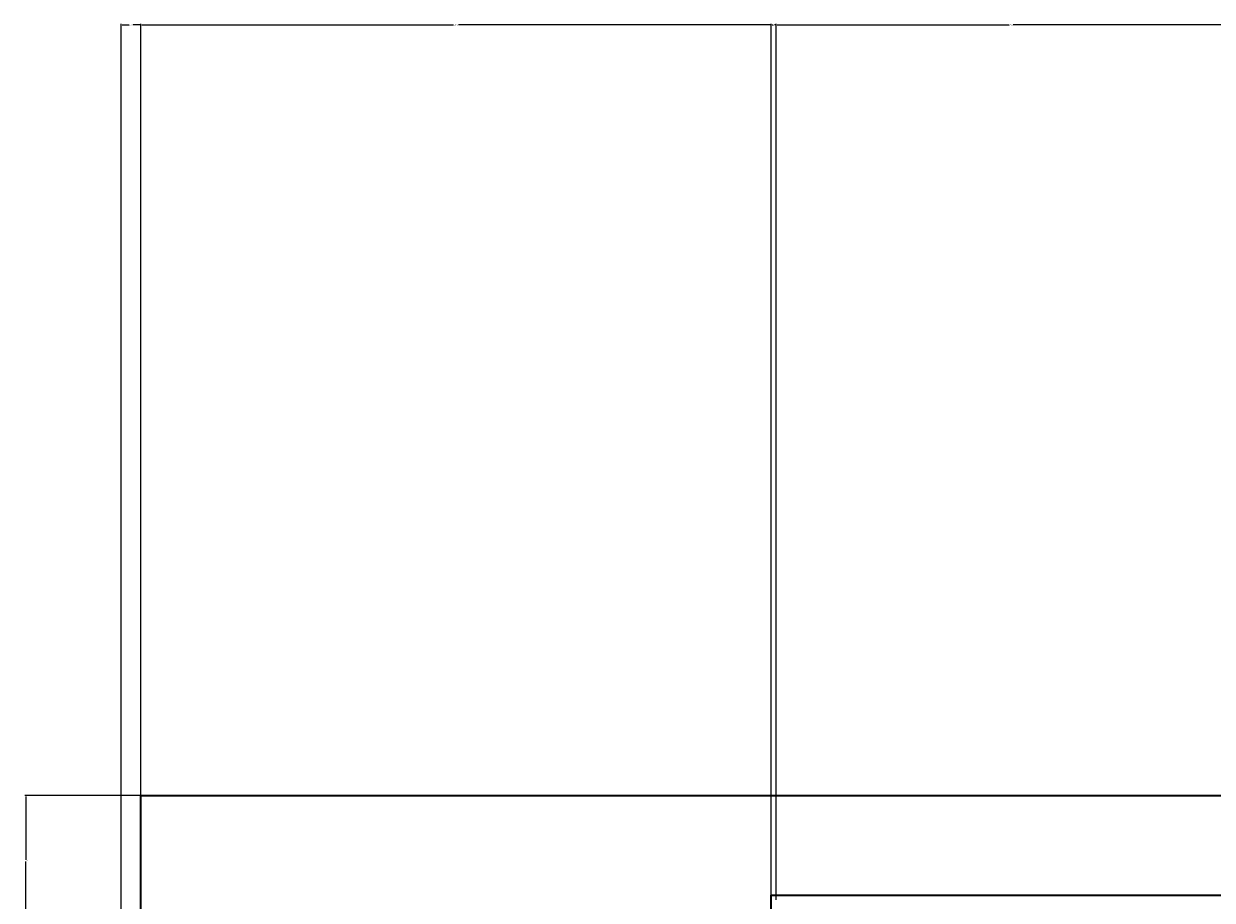
# Model space of a CAD drawing. Units: inches. Extents: x -7 to 391, y -12 to 303.
# Tile 2 of 5: x -7 to 222, y 134 to 303. Entities that reach past the tile are written whole.
import ezdxf

# ---------------------------------------------------------------- set-up
doc = ezdxf.new("R2010")
doc.units = ezdxf.units.IN
doc.header["$MEASUREMENT"] = 0
doc.layers.add('A-ANNO-DIMS', color=2, linetype='Continuous', lineweight=18)
doc.layers.add('A-ELEV', color=7, linetype='Continuous', lineweight=35)
doc.styles.get("Standard").update_dxf_attribs({"font": 'arial.ttf'})
doc.dimstyles.get("Standard").update_dxf_attribs({"dimtxt": 0.18, "dimasz": 0.18, "dimexe": 0.18, "dimexo": 0.0625, "dimgap": 0.09, "dimtad": 0, "dimtih": 1, "dimtoh": 1, "dimdec": 4, "dimzin": 0, "dimdsep": 46, "dimtxsty": 'Standard', "dimcen": 0.09, "dimadec": 0, "dimazin": 0, "dimtfac": 1, "dimtdec": 4, "dimtofl": 0, "dimtmove": 0, "dimatfit": 3, "dimfxl": 1, "dimtolj": 1, "dimtzin": 0, "dimarcsym": 0})

# ---------------------------------------------------------------- blocks, each defined once
blk = doc.blocks.new('*D16')
at = {"layer": 'A-ANNO-DIMS', "color": 0, "lineweight": -2, "transparency": 16777216}
for p, q in [((15.76, 154.35), (-6.56, 154.35)), ((-6.38, 154.17), (-6.38, 141.98)), ((-6.38, 129.43), (-6.38, 141.62)), ((11.96, 129.25), (-6.56, 129.25))]:
    blk.add_line(p, q, dxfattribs=at)
at = {"layer": 'A-ANNO-DIMS', "color": 0, "transparency": 16777216}
for points in [[(-6.41, 154.17), (-6.35, 154.17), (-6.38, 154.35)], [(-6.41, 129.43), (-6.35, 129.43), (-6.38, 129.25)]]:
    blk.add_solid(points, dxfattribs=at)
at = {"layer": 'Defpoints', "color": 0, "transparency": 16777216}
for p in [(-6.38, 154.35), (15.82, 154.35), (12.02, 129.25)]:
    blk.add_point(p, dxfattribs=at)
at = {"layer": 'A-ANNO-DIMS', "color": 0, "transparency": 16777216, "insert": (-6.38, 141.8), "char_height": 0.18, "attachment_point": 5}
blk.add_mtext('\\A1;25.095', dxfattribs=at)
blk = doc.blocks.new('*D18')
at = {"layer": 'A-ANNO-DIMS', "color": 0, "lineweight": -2, "transparency": 16777216}
for p, q in [((12.02, 129.31), (12.02, 303.01)), ((12.2, 302.83), (13.53, 302.83)), ((15.64, 302.83), (14.31, 302.83)), ((15.82, 154.41), (15.82, 303.01))]:
    blk.add_line(p, q, dxfattribs=at)
at = {"layer": 'A-ANNO-DIMS', "color": 0, "transparency": 16777216}
for points in [[(12.2, 302.86), (12.2, 302.8), (12.02, 302.83)], [(15.64, 302.86), (15.64, 302.8), (15.82, 302.83)]]:
    blk.add_solid(points, dxfattribs=at)
at = {"layer": 'Defpoints', "color": 0, "transparency": 16777216}
for p in [(15.82, 302.83), (15.82, 154.35), (12.02, 129.25)]:
    blk.add_point(p, dxfattribs=at)
at = {"layer": 'A-ANNO-DIMS', "color": 0, "transparency": 16777216, "insert": (13.92, 302.83), "char_height": 0.18, "attachment_point": 5}
blk.add_mtext('\\A1;3.799', dxfattribs=at)
blk = doc.blocks.new('*D19')
at = {"layer": 'A-ANNO-DIMS', "color": 0, "lineweight": -2, "transparency": 16777216}
for p, q in [((15.82, 154.41), (15.82, 303.01)), ((16, 302.83), (76.08, 302.83)), ((137.06, 302.83), (76.99, 302.83)), ((137.24, 135.24), (137.24, 303.01))]:
    blk.add_line(p, q, dxfattribs=at)
at = {"layer": 'A-ANNO-DIMS', "color": 0, "transparency": 16777216}
for points in [[(16, 302.86), (16, 302.8), (15.82, 302.83)], [(137.06, 302.86), (137.06, 302.8), (137.24, 302.83)]]:
    blk.add_solid(points, dxfattribs=at)
at = {"layer": 'Defpoints', "color": 0, "transparency": 16777216}
for p in [(137.24, 302.83), (15.82, 154.35), (137.24, 135.18)]:
    blk.add_point(p, dxfattribs=at)
at = {"layer": 'A-ANNO-DIMS', "color": 0, "transparency": 16777216, "insert": (76.53, 302.83), "char_height": 0.18, "attachment_point": 5}
blk.add_mtext('\\A1;121.42', dxfattribs=at)
blk = doc.blocks.new('*D20')
at = {"layer": 'A-ANNO-DIMS', "color": 0, "lineweight": -2, "transparency": 16777216}
for p, q in [((137.24, 135.24), (137.24, 303.01)), ((137.42, 302.83), (137.62, 302.83)), ((138.06, 302.83), (137.87, 302.83)), ((138.24, 134.24), (138.24, 303.01))]:
    blk.add_line(p, q, dxfattribs=at)
at = {"layer": 'A-ANNO-DIMS', "color": 0, "transparency": 16777216}
for points in [[(137.42, 302.86), (137.42, 302.8), (137.24, 302.83)], [(138.06, 302.86), (138.06, 302.8), (138.24, 302.83)]]:
    blk.add_solid(points, dxfattribs=at)
at = {"layer": 'Defpoints', "color": 0, "transparency": 16777216}
for p in [(138.24, 302.83), (137.24, 135.18), (138.24, 134.18)]:
    blk.add_point(p, dxfattribs=at)
at = {"layer": 'A-ANNO-DIMS', "color": 0, "transparency": 16777216, "insert": (137.74, 302.83), "char_height": 0.18, "attachment_point": 5}
blk.add_mtext('\\A1;1', dxfattribs=at)
blk = doc.blocks.new('*D21')
at = {"layer": 'A-ANNO-DIMS', "color": 0, "lineweight": -2, "transparency": 16777216}
for p, q in [((138.24, 134.24), (138.24, 303.01)), ((138.42, 302.83), (183.11, 302.83)), ((228.58, 302.83), (183.89, 302.83)), ((228.76, 284.49), (228.76, 303.01))]:
    blk.add_line(p, q, dxfattribs=at)
at = {"layer": 'A-ANNO-DIMS', "color": 0, "transparency": 16777216}
for points in [[(138.42, 302.86), (138.42, 302.8), (138.24, 302.83)], [(228.58, 302.86), (228.58, 302.8), (228.76, 302.83)]]:
    blk.add_solid(points, dxfattribs=at)
at = {"layer": 'Defpoints', "color": 0, "transparency": 16777216}
for p in [(228.76, 302.83), (228.76, 284.43), (138.24, 134.18)]:
    blk.add_point(p, dxfattribs=at)
at = {"layer": 'A-ANNO-DIMS', "color": 0, "transparency": 16777216, "insert": (183.5, 302.83), "char_height": 0.18, "attachment_point": 5}
blk.add_mtext('\\A1;90.52', dxfattribs=at)

msp = doc.modelspace()

# ---------------------------------------------------------------- linework, layer by layer
at = {"layer": 'A-ELEV'}
for p, q in [((15.8204, 154.3452), (372.0212, 154.3452)), ((15.8204, 129.2504), (15.8204, 154.3452)), ((137.2426, 6.3452), (137.2426, 135.1767)), ((137.2426, 135.1767), (372.0212, 135.1767))]:
    msp.add_line(p, q, dxfattribs=at)

# ---------------------------------------------------------------- dimensions: what is measured, and where the dimension line sits
at = {"layer": 'A-ANNO-DIMS'}
for base, p1, p2, override, picture, middle in [((15.8204, 302.832), (12.0212, 129.2504), (15.8204, 154.3452), {"dimdec": 3, "dimlfac": 1, "dimrnd": 0, "dimzin": 0, "dimdsep": 46, "dimlunit": 2}, '*D18', (13.9208, 302.832)), ((137.2426, 302.832), (15.8204, 154.3452), (137.2426, 135.1767), {"dimdec": 2, "dimlfac": 1, "dimrnd": 0, "dimzin": 0, "dimdsep": 46, "dimlunit": 2}, '*D19', (76.5315, 302.832)), ((138.2426, 302.832), (137.2426, 135.1767), (138.2426, 134.1767), {"dimdec": 0, "dimlfac": 1, "dimrnd": 0, "dimzin": 0, "dimdsep": 46, "dimlunit": 2}, '*D20', (137.7426, 302.832)), ((228.758, 302.832), (138.2426, 134.1767), (228.758, 284.432), {"dimdec": 2, "dimlfac": 1, "dimrnd": 0, "dimzin": 0, "dimdsep": 46, "dimlunit": 2}, '*D21', (183.5003, 302.832))]:
    dim = msp.add_linear_dim(base=base, p1=p1, p2=p2, dimstyle='Standard', override=override, dxfattribs=at)
    dim.commit()
    dim.dimension.update_dxf_attribs({"geometry": picture, "text_midpoint": middle})
dim = msp.add_linear_dim(base=(-6.3788, 154.3452), p1=(12.0212, 129.2504), p2=(15.8204, 154.3452), angle=90, dimstyle='Standard', override={"dimdec": 3, "dimlfac": 1, "dimrnd": 0, "dimzin": 0, "dimdsep": 46, "dimlunit": 2}, dxfattribs=at)
dim.commit()
dim.dimension.update_dxf_attribs({"geometry": '*D16', "text_midpoint": (-6.3788, 141.7978)})

doc.saveas('drawing.dxf')
